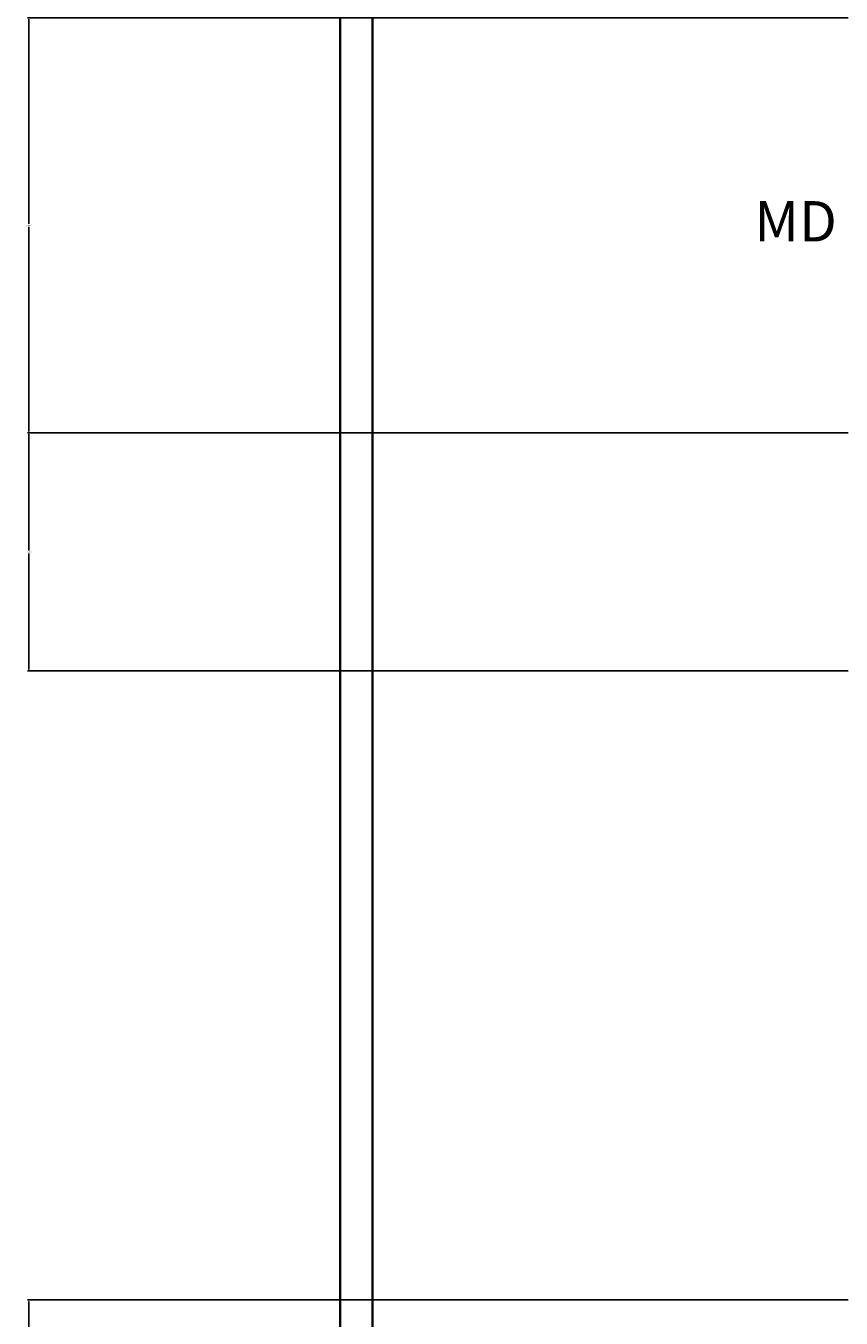
# Model space of a CAD drawing. Units: inches. Extents: x -86 to 2463, y -1058 to 68.
# Tile 3 of 17: x -86 to 15, y -383 to -223. Entities that reach past the tile are written whole.
import ezdxf

# ---------------------------------------------------------------- set-up
doc = ezdxf.new("R2010")
doc.units = ezdxf.units.IN
doc.header["$MEASUREMENT"] = 0
for name, color, linetype, lineweight in [('A-ANNO-DIMS', 2, 'Continuous', 18), ('A-ANNO-TEXT', 7, 'Continuous', 18), ('A-WALL', 7, 'Continuous', 35)]:
    doc.layers.add(name, color=color, linetype=linetype, lineweight=lineweight)
doc.styles.get("Standard").update_dxf_attribs({"font": 'arial.ttf'})
doc.dimstyles.get("Standard").update_dxf_attribs({"dimtxt": 0.18, "dimasz": 0.18, "dimexe": 0.18, "dimexo": 0.0625, "dimgap": 0.09, "dimtad": 0, "dimtih": 1, "dimtoh": 1, "dimdec": 4, "dimzin": 0, "dimdsep": 46, "dimtxsty": 'Standard', "dimcen": 0.09, "dimadec": 0, "dimazin": 0, "dimtfac": 1, "dimtdec": 4, "dimtofl": 0, "dimtmove": 0, "dimatfit": 3, "dimfxl": 1, "dimtolj": 1, "dimtzin": 0, "dimarcsym": 0})

# ---------------------------------------------------------------- blocks, each defined once
blk = doc.blocks.new('*D33')
at = {"layer": 'A-ANNO-DIMS', "color": 0, "lineweight": -2, "transparency": 16777216}
for p, q in [((15.7, -381.1), (-86.02, -381.1)), ((-85.84, -381.28), (-85.84, -504.09)), ((-85.84, -627.25), (-85.84, -504.45)), ((15.7, -627.43), (-86.02, -627.43))]:
    blk.add_line(p, q, dxfattribs=at)
at = {"layer": 'A-ANNO-DIMS', "color": 0, "transparency": 16777216}
for points in [[(-85.87, -381.28), (-85.81, -381.28), (-85.84, -381.1)], [(-85.87, -627.25), (-85.81, -627.25), (-85.84, -627.43)]]:
    blk.add_solid(points, dxfattribs=at)
at = {"layer": 'Defpoints', "color": 0, "transparency": 16777216}
for p in [(-85.84, -381.1), (15.76, -381.1), (15.76, -627.43)]:
    blk.add_point(p, dxfattribs=at)
at = {"layer": 'A-ANNO-DIMS', "color": 0, "transparency": 16777216, "insert": (-85.84, -504.27), "char_height": 0.18, "attachment_point": 5}
blk.add_mtext('\\A1;246.33', dxfattribs=at)
blk = doc.blocks.new('*D37')
at = {"layer": 'A-ANNO-DIMS', "color": 0, "lineweight": -2, "transparency": 16777216}
for p, q in [((15.7, -273.57), (-86.02, -273.57)), ((-85.84, -273.75), (-85.84, -288.16)), ((-85.84, -302.92), (-85.84, -288.52)), ((15.7, -303.1), (-86.02, -303.1))]:
    blk.add_line(p, q, dxfattribs=at)
at = {"layer": 'A-ANNO-DIMS', "color": 0, "transparency": 16777216}
for points in [[(-85.87, -273.75), (-85.81, -273.75), (-85.84, -273.57)], [(-85.87, -302.92), (-85.81, -302.92), (-85.84, -303.1)]]:
    blk.add_solid(points, dxfattribs=at)
at = {"layer": 'Defpoints', "color": 0, "transparency": 16777216}
for p in [(-85.84, -273.57), (15.76, -273.57), (15.76, -303.1)]:
    blk.add_point(p, dxfattribs=at)
at = {"layer": 'A-ANNO-DIMS', "color": 0, "transparency": 16777216, "insert": (-85.84, -288.34), "char_height": 0.18, "attachment_point": 5}
blk.add_mtext('\\A1;29.53', dxfattribs=at)
blk = doc.blocks.new('*D38')
at = {"layer": 'A-ANNO-DIMS', "color": 0, "lineweight": -2, "transparency": 16777216}
for p, q in [((15.7, -222.1), (-86.02, -222.1)), ((-85.84, -222.28), (-85.84, -247.66)), ((-85.84, -273.39), (-85.84, -248.02)), ((15.7, -273.57), (-86.02, -273.57))]:
    blk.add_line(p, q, dxfattribs=at)
at = {"layer": 'A-ANNO-DIMS', "color": 0, "transparency": 16777216}
for points in [[(-85.87, -222.28), (-85.81, -222.28), (-85.84, -222.1)], [(-85.87, -273.39), (-85.81, -273.39), (-85.84, -273.57)]]:
    blk.add_solid(points, dxfattribs=at)
at = {"layer": 'Defpoints', "color": 0, "transparency": 16777216}
for p in [(-85.84, -222.1), (15.76, -222.1), (15.76, -273.57)]:
    blk.add_point(p, dxfattribs=at)
at = {"layer": 'A-ANNO-DIMS', "color": 0, "transparency": 16777216, "insert": (-85.84, -247.84), "char_height": 0.18, "attachment_point": 5}
blk.add_mtext('\\A1;51.47', dxfattribs=at)

msp = doc.modelspace()

# ---------------------------------------------------------------- linework, layer by layer
at = {"layer": 'A-WALL'}
for p, q in [((-47.239, -141.104), (-47.239, -701.604)), ((-43.239, -141.104), (-43.239, -697.604))]:
    msp.add_line(p, q, dxfattribs=at)

# ---------------------------------------------------------------- texts
at = {"layer": 'A-ANNO-TEXT', "insert": (4.075, -244.841), "char_height": 5, "attachment_point": 1}
msp.add_mtext_dynamic_manual_height_columns('MD ', width=17.85419, gutter_width=25, heights=[0], dxfattribs=at)

# ---------------------------------------------------------------- dimensions: what is measured, and where the dimension line sits
at = {"layer": 'A-ANNO-DIMS'}
for base, p1, p2, picture, middle in [((-85.839, -222.104), (15.761, -273.574), (15.761, -222.104), '*D38', (-85.839, -247.839)), ((-85.839, -273.574), (15.761, -303.104), (15.761, -273.574), '*D37', (-85.839, -288.339)), ((-85.839, -381.104), (15.761, -627.432), (15.761, -381.104), '*D33', (-85.839, -504.268))]:
    dim = msp.add_linear_dim(base=base, p1=p1, p2=p2, angle=90, dimstyle='Standard', override={"dimdec": 2, "dimlfac": 1, "dimrnd": 0, "dimzin": 0, "dimdsep": 46, "dimlunit": 2}, dxfattribs=at)
    dim.commit()
    dim.dimension.update_dxf_attribs({"geometry": picture, "text_midpoint": middle})

doc.saveas('drawing.dxf')
